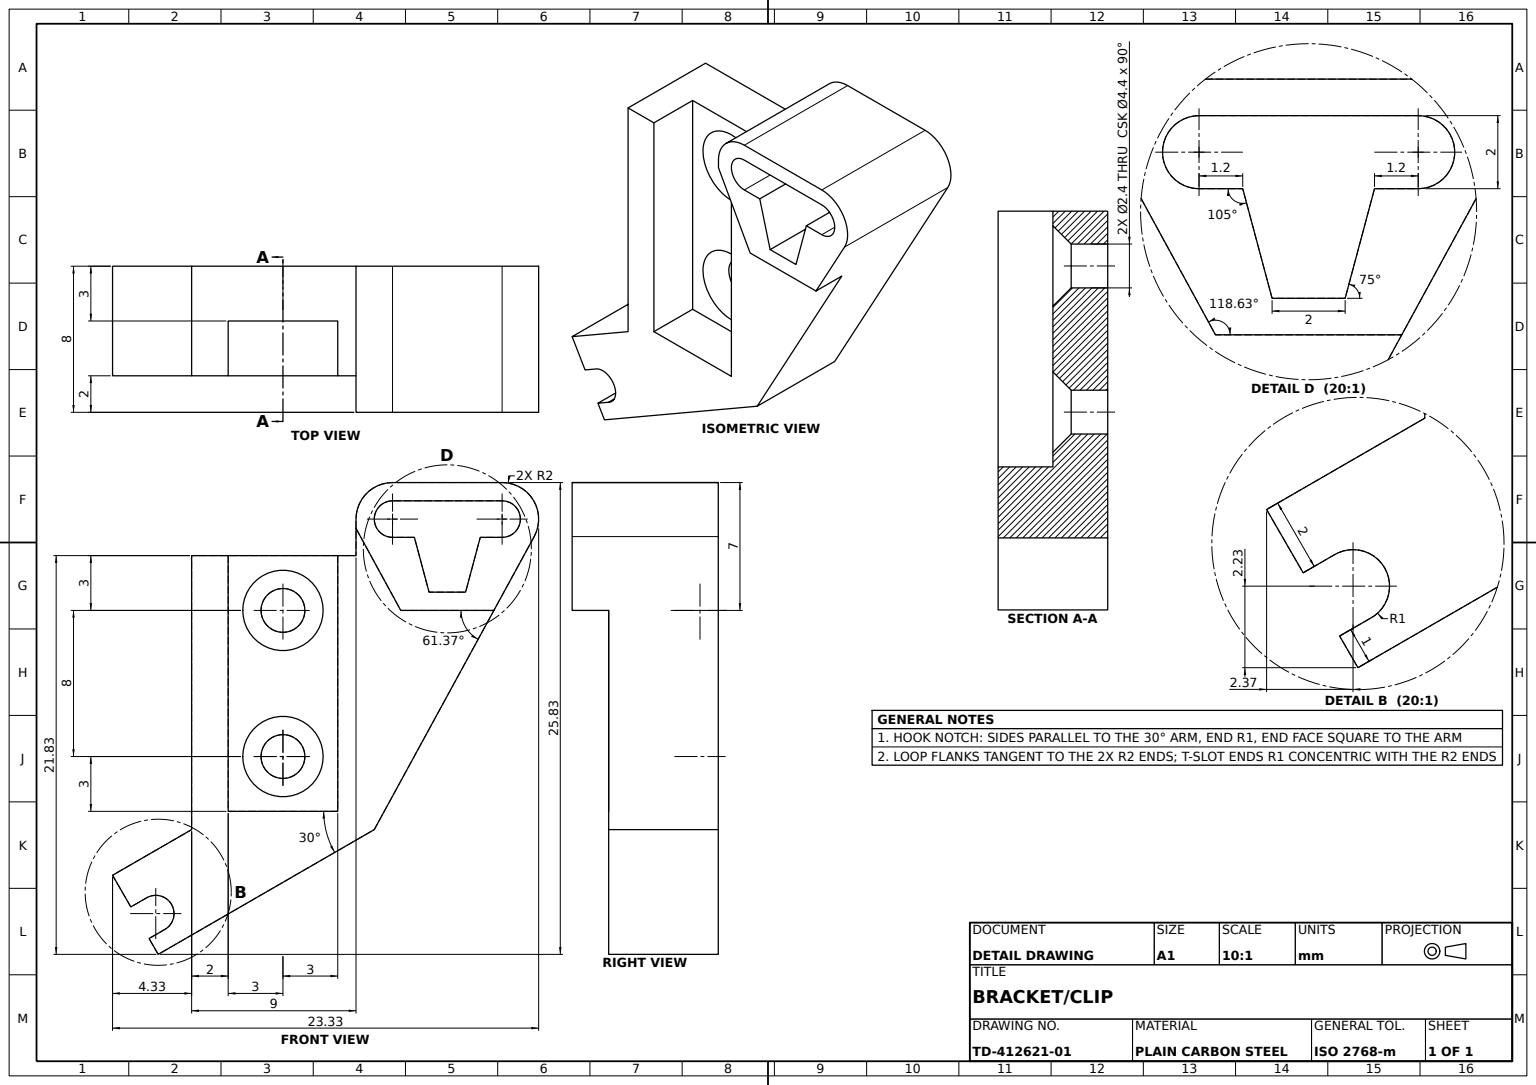
from build123d import *

# Parameters (mm, degrees)
L_BRACKET_BODY_DEPTH             = 6
TRAPEZOID_SLOT_BOSS_DEPTH        = 2
POCKET_CUT_DEPTH                 = 14
M2_COUNTERSUNK_HOLES_D           = 2.4
M2_COUNTERSUNK_HOLES_CSINK_D     = 4.4
M2_COUNTERSUNK_HOLES_CSINK_ANGLE = 90


with BuildPart() as part:
    # L Bracket Profile Sketch → L Bracket Body (new body)
    # profile 1 of 2: a face of its own
    with BuildSketch(Plane.XY):
        with BuildLine():
            Line((0, 15), (0, 0))
            Line((0, 0), (-4.330127019, -2.5))
            Line((-4.330127019, -2.5), (-3.329569645, -4.233016207))
            Line((-3.329569645, -4.233016207), (-2.504424414, -3.756618386))
            ThreePointArc((-2.504424414, -3.756618386), (-1.098076211, -4.098076211), (-1.505539161, -5.486738395))
            Line((-1.505539161, -5.486738395), (-2.330684392, -5.963136216))
            Line((-2.330684392, -5.963136216), (-1.830127019, -6.830127019))
            Line((-1.830127019, -6.830127019), (10, 0))
            Line((10, 0), (16.549529843, 12))
            Line((16.549529843, 12), (14, 12))
            Line((14, 12), (11.450470157, 12))
            Line((11.450470157, 12), (9.244459544, 16.041836283))
            ThreePointArc((9.244459544, 16.041836283), (9.062078315, 16.505571497), (9, 17))
            Line((9, 17), (9, 15))
            Line((9, 15), (0, 15))
        make_face()
    # profile 2 of 2: a face of its own
    with BuildSketch(Plane.XY):
        with BuildLine():
            ThreePointArc((11, 19), (9.585786438, 18.414213562), (9, 17))
            ThreePointArc((9, 17), (9.062078315, 16.505571497), (9.244459544, 16.041836283))
            Line((9.244459544, 16.041836283), (11.450470157, 12))
            Line((11.450470157, 12), (14, 12))
            Line((14, 12), (16.549529843, 12))
            Line((16.549529843, 12), (18.755540456, 16.041836283))
            ThreePointArc((18.755540456, 16.041836283), (18.719931312, 18.020703817), (17, 19))
            Line((17, 19), (11, 19))
        make_face()
        with BuildLine():
            Line((15, 13), (13, 13))
            Line((13, 13), (12.196152423, 16))
            Line((12.196152423, 16), (11, 16))
            ThreePointArc((11, 16), (10, 17), (11, 18))
            Line((11, 18), (17, 18))
            ThreePointArc((17, 18), (18, 17), (17, 16))
            Line((17, 16), (15.803847577, 16))
            Line((15.803847577, 16), (15, 13))
        make_face(mode=Mode.SUBTRACT)
    extrude(amount=L_BRACKET_BODY_DEPTH)

    # Trapezoid Slot Boss Sketch → Trapezoid Slot Boss (add)
    with BuildSketch(Plane.XY.offset(6)):
        with BuildLine():
            Line((14, 12), (16.549529843, 12))
            Line((16.549529843, 12), (18.755540456, 16.041836283))
            ThreePointArc((18.755540456, 16.041836283), (18.719931312, 18.020703817), (17, 19))
            Line((17, 19), (11, 19))
            ThreePointArc((11, 19), (9.585786438, 18.414213562), (9, 17))
            Line((9, 17), (9, 16.489733247))
            Line((9, 16.489733247), (11.450470157, 12))
            Line((11.450470157, 12), (14, 12))
        make_face()
        with BuildLine():
            Line((11, 18), (17, 18))
            ThreePointArc((17, 18), (18, 17), (17, 16))
            Line((17, 16), (15.803847577, 16))
            Line((15.803847577, 16), (15, 13))
            Line((15, 13), (13, 13))
            Line((13, 13), (12.196152423, 16))
            Line((12.196152423, 16), (11, 16))
            ThreePointArc((11, 16), (10, 17), (11, 18))
        make_face(mode=Mode.SUBTRACT)
    extrude(amount=TRAPEZOID_SLOT_BOSS_DEPTH)

    # Pocket Cut Sketch → Pocket Cut (cut)
    with BuildSketch(Plane(origin=(0, 15, 0), x_dir=(1, 0, 0), z_dir=(0, 1, 0))):
        Polygon((2, -3), (2, -6), (5, -6), (8, -6), (8, -3), (5, -3), align=None)
    extrude(amount=-POCKET_CUT_DEPTH, mode=Mode.SUBTRACT)

    # M2 Countersunk Holes (through all)
    with Locations(Plane.XY.offset(3)):
        with Locations((5, 12), (5, 4)):
            CounterSinkHole(M2_COUNTERSUNK_HOLES_D / 2, M2_COUNTERSUNK_HOLES_CSINK_D / 2, counter_sink_angle=M2_COUNTERSUNK_HOLES_CSINK_ANGLE)


solid = part.part
